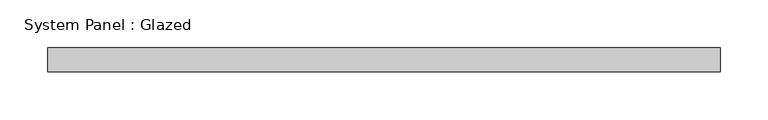
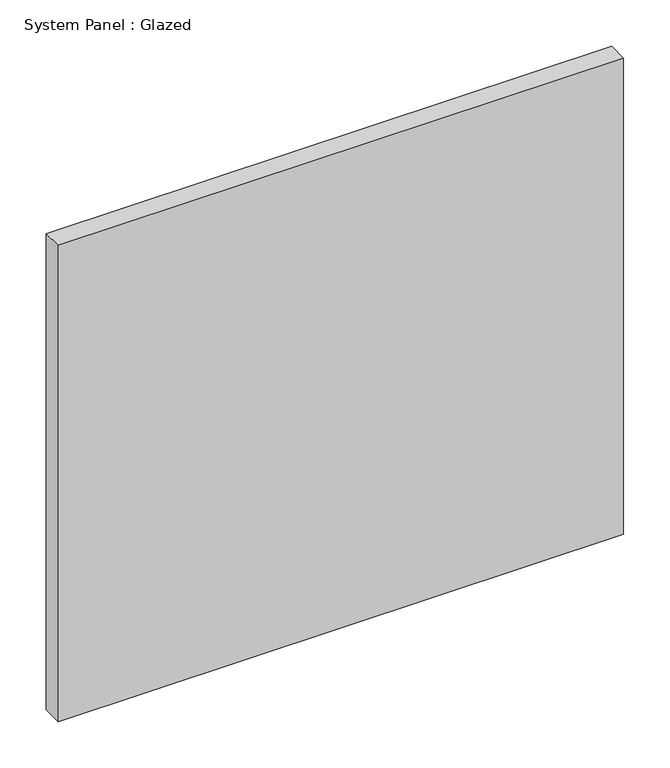
"""IFC4 building model written with IfcOpenShell, lengths in millimetres: plate geometry, System Panel : Glazed."""

from ifc_helpers import new_model, si_unit, origin, origin_with_axes, place, context, project, spatial, polyline, outline, extrude, source, transform, mapped, element, save


def system_panel_glazed_daf883b7(model_context):
    return source(origin(), model_context, "Body", "SweptSolid", [
        extrude(outline(polyline([(352.4140615, 19.05), (-352.4140615, 19.05), (-352.4140615, 44.45), (352.4140615, 44.45), (352.4140615, 19.05)])), origin_with_axes(), (0.0, 0.0, 1.0), 627.1281505),
    ])


if __name__ == "__main__":
    model = new_model("IFC4")
    model_context = context("Model", 3, world=origin())
    ifc_project = project(units=[si_unit("LENGTHUNIT", "METRE", prefix="MILLI")], contexts=[model_context])
    site = spatial("IfcSite", under=ifc_project)
    building = spatial("IfcBuilding", under=site)
    placement = place(None, origin())
    system_panel_glazed_shape = system_panel_glazed_daf883b7(model_context)
    element("IfcPlate", 1, ObjectType="System Panel : Glazed", at=placement, inside=building, context=model_context, shape_type="MappedRepresentation", body=[
        mapped(system_panel_glazed_shape, transform((0.0, 0.0, 0.0), x_axis=(1.0, 0.0, 0.0), y_axis=(0.0, 1.0, 0.0), z_axis=(0.0, 0.0, 1.0))),
    ])
    save(model, "model.ifc")

# Revit data of these elements
# Type "System Panel : Glazed"
#   Construction Type Id = "GSP4R"
#   Analytic Construction = "1/8 in Pilkington single glazing"
#   Visual Light Transmittance = 0.9
#   Solar Heat Gain Coefficient = 0.86
#   Heat Transfer Coefficient (U) = 1.18115 BTU/(h·ft²·°F)
#   Define Thermal Properties by = 1
# Element 1 (IfcPlate, "System Panel : Glazed")
#   Materials on its faces: "Glass"
# Materials
#   "Glass": class "Glass", colour RGB 0 128 192, transparency 0.75, Description = "Soda Lime Glass", Cost = 0
